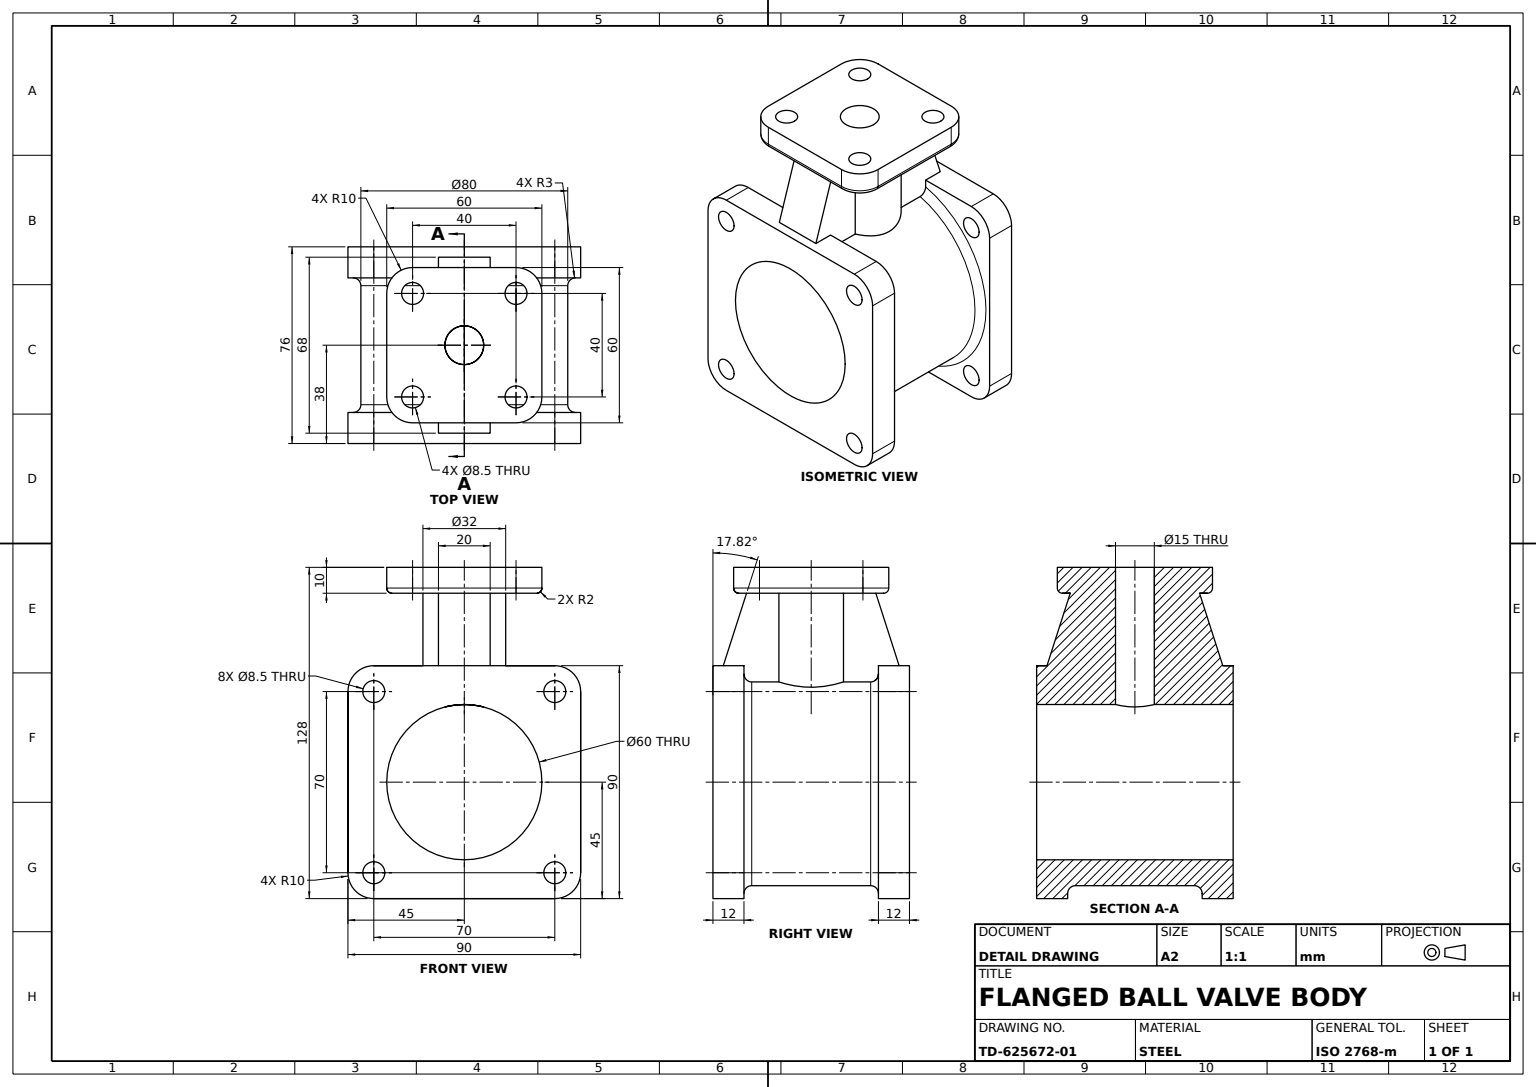
SolidWorks part; units mm, degrees
material "Plain Carbon Steel"
ref_plane "Front Plane" through (0, 0, 0) normal (0, 0, 1) x (1, 0, 0)
ref_plane "Top Plane" through (0, 0, 0) normal (0, 1, 0) x (1, 0, 0)
ref_plane "Right Plane" through (0, 0, 0) normal (1, 0, 0) x (0, 0, -1)
sketch "Body Tube Sketch" plane through (0, 0, 0) normal (1, 0, 0) x (0, 0, -1)
  circle A0 centre (0, 0) radius 40
  circle A1 centre (0, 0) radius 30
  dimension "D1" = 80
  dimension "D2" = 60
extrude "Body Tube" add sketch "Body Tube Sketch" along normal blind 76
sketch "End Flange Sketch" plane through (0, 0, 0) normal (-1, 0, 0) x (0, 0, 1)
  line L1 (-35, -45) -> (35, -45)
  line L2 (-45, -35) -> (-45, 35)
  line L3 (-35, 45) -> (35, 45)
  line L4 (45, -35) -> (45, 35)
  line L5 (-45, -45) -> (45, 45) construction
  line L6 (-45, 45) -> (45, -45) construction
  arc A0 (-35, -45) -> (-45, -35) centre (-35, -35) cw
  arc A1 (35, -45) -> (45, -35) centre (35, -35) ccw
  arc A2 (35, 45) -> (45, 35) centre (35, 35) cw
  arc A3 (-45, 35) -> (-35, 45) centre (-35, 35) cw
  point P0 (0, 0)
  dimension "D3" = 10
  dimension "D1" = 90
  dimension "D2" = 90
extrude "End Flange" add sketch "End Flange Sketch" against normal blind 12
sketch "Body Bore Sketch" plane through (0, 0, 0) normal (-1, 0, 0) x (0, 0, 1)
  circle A1 centre (0, 0) radius 30
  circle A2 centre (0, 0) radius 30
  dimension "D1" = 0
extrude "Body Bore Ø60" cut sketch "Body Bore Sketch" against normal through all
sketch "End Flange Bolt Holes Sketch" plane through (0, 0, 0) normal (-1, 0, 0) x (0, 0, 1)
  circle A0 centre (-35, 35) radius 4.25
  circle A1 centre (35, 35) radius 4.25
  circle A2 centre (-35, -35) radius 4.25
  circle A3 centre (35, -35) radius 4.25
  dimension "D1" = 8.5
  dimension "D2" = 8.5
  dimension "D3" = 8.5
  dimension "D4" = 8.5
extrude "End Flange Bolt Holes 4xØ8.5" cut sketch "End Flange Bolt Holes Sketch" against normal blind 12
ref_plane "Body Mid Plane" through (38, 0, 0) normal (1, 0, 0) x (0, 0, -1)
mirror "Opposite End Flange Mirror" about plane through (38, 0, 0) normal (1, 0, 0) of "End Flange"
mirror "Opposite Flange Holes and Bore Mirror" about plane through (38, 0, 0) normal (1, 0, 0) of "End Flange Bolt Holes 4xØ8.5", "Body Bore Ø60"
ref_plane "Top Flange Plane" through (0, 83, 0) normal (0, 1, 0) x (1, 0, 0)
sketch "Top Flange Sketch" plane through (0, 83, 0) normal (0, 1, 0) x (1, 0, 0)
  line L1 (18, -30) -> (58, -30)
  line L2 (8, -20) -> (8, 20)
  line L3 (18, 30) -> (58, 30)
  line L4 (68, -20) -> (68, 20)
  line L5 (8, -30) -> (68, 30) construction
  line L6 (8, 30) -> (68, -30) construction
  arc A0 (18, -30) -> (8, -20) centre (18, -20) cw
  arc A1 (58, -30) -> (68, -20) centre (58, -20) ccw
  arc A2 (58, 30) -> (68, 20) centre (58, 20) cw
  arc A3 (8, 20) -> (18, 30) centre (18, 20) cw
  point P0 (38, 0)
  dimension "D5" = 10
  dimension "D1" = 60
  dimension "D2" = 60
  dimension "D3" = 30
  dimension "D4" = 38
extrude "Top Flange" add sketch "Top Flange Sketch" against normal blind 10 separate body
sketch "Stem Neck Sketch" plane through (0, 83, 0) normal (0, 1, 0) x (1, 0, 0)
  line L0 (58, 30) -> (18, 30) construction
  circle A0 centre (38, 0) radius 16
  dimension "D1" = 32
  dimension "D2" = 38
  dimension "D3" = 30
extrude "Stem Neck Ø32" add sketch "Stem Neck Sketch" against normal blind 48
ref_plane "Rib Sketch Plane" through (0, 0, 0) normal (0, 0, 1) x (1, 0, 0)
sketch "Neck Support Rib Sketch" plane through (0, 0, 0) normal (0, 0, 1) x (1, 0, 0)
  line L0 (27.2291, 73) -> (27.2291, 33)
  line L1 (18, 73) -> (58, 73) construction
  line L2 (27.2291, 33) -> (12, 33)
  line L3 (12, -40) -> (12, 40) construction
  line L4 (12, 33) -> (12, 45)
  line L5 (12, 35) -> (12, 45) construction
  line L6 (12, 45) -> (4, 45)
  line L7 (12, 45) -> (0, 45) construction
  line L8 (4, 45) -> (13, 73)
  line L9 (8, 73) -> (18, 73) construction
  line L10 (13, 73) -> (27.2291, 73)
  dimension "D1" = 40
  dimension "D2" = 8
  dimension "D3" = 15.2291
  dimension "D4" = 12
extrude "Neck Support Rib" add sketch "Neck Support Rib Sketch" along normal mid plane 20
ref_plane "Rib Mirror Plane" through (38, 0, 0) normal (1, 0, 0) x (0, 0, -1)
mirror "Neck Support Rib Mirror" about plane through (38, 0, 0) normal (1, 0, 0) of "Neck Support Rib"
sketch "Top Flange Bolt Holes Sketch" plane through (0, 83, 0) normal (0, 1, 0) x (1, 0, 0)
  circle A0 centre (18, 20) radius 4.25
  circle A1 centre (58, 20) radius 4.25
  circle A2 centre (18, -20) radius 4.25
  circle A3 centre (58, -20) radius 4.25
  dimension "D1" = 8.5
  dimension "D2" = 8.5
  dimension "D3" = 8.5
  dimension "D4" = 8.5
extrude "Top Flange Bolt Holes 4xØ8.5" cut sketch "Top Flange Bolt Holes Sketch" against normal blind 20
sketch "Stem Bore Sketch" plane through (0, 83, 0) normal (0, 1, 0) x (1, 0, 0)
  line L0 (18, -30) -> (58, -30) construction
  circle A0 centre (38, 0) radius 7.5
  dimension "D1" = 15
  dimension "D2" = 38
  dimension "D3" = 30
extrude "Stem Bore Ø15" cut sketch "Stem Bore Sketch" against normal blind 54
fillet "End Flange Fillets R3" radius 3 2 edges at (64, -40, 0) (12, -40, 0)
fillet "Top Flange Fillets R2" radius 2 8 edges at (8, 73, 0) (10.9289, 73, -27.0711) (38, 73, -30) (65.0711, 73, -27.0711) (68, 73, 0) (65.0711, 73, 27.0711) (38, 73, 30) (10.9289, 73, 27.0711)
